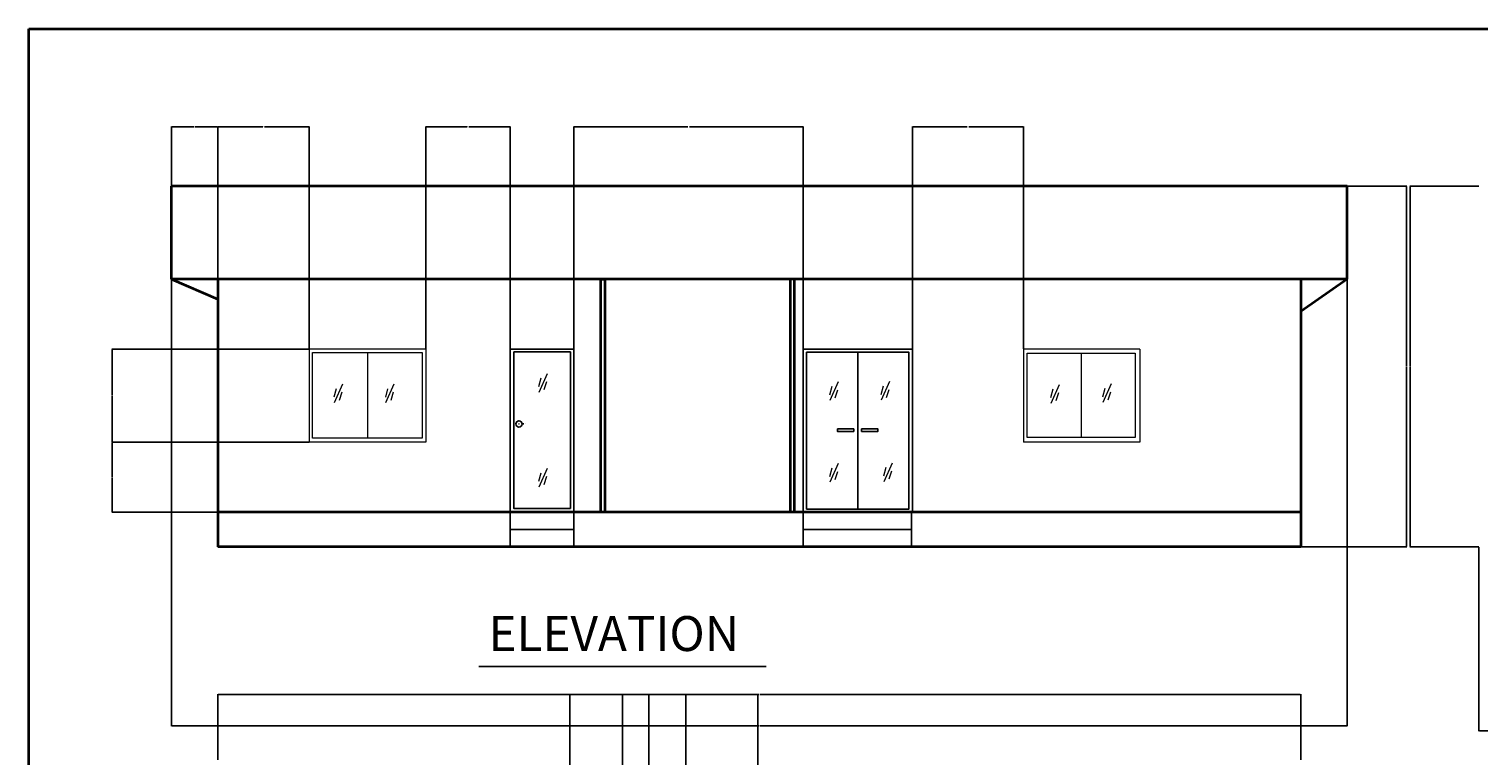
# Model space of a CAD drawing. Units: inches. Extents: x 2215 to 3724, y 1009 to 2124.
# Tile 7 of 11: x 2215 to 2963, y 1750 to 2124. Entities that reach past the tile are written whole.
import ezdxf

# ---------------------------------------------------------------- set-up
doc = ezdxf.new("R2010")
doc.units = ezdxf.units.IN
for name, color, linetype, lineweight in [('A-ANNO-DIMS', 2, 'Continuous', 18), ('A-ANNO-TEXT', 7, 'Continuous', 25), ('A-ANNO-TTLB', 7, 'Continuous', 35), ('A-DOOR', 3, 'Continuous', 25), ('A-ELEV', 7, 'Continuous', 35), ('A-FLOR-STRS', 7, 'Continuous', 25), ('A-GLAZ', 4, 'Continuous', 18)]:
    doc.layers.add(name, color=color, linetype=linetype, lineweight=lineweight)
doc.styles.get("Standard").update_dxf_attribs({"font": 'arial.ttf'})
doc.dimstyles.get("Standard").update_dxf_attribs({"dimtxt": 0.18, "dimasz": 0.18, "dimexe": 0.18, "dimexo": 0.0625, "dimgap": 0.09, "dimtad": 0, "dimtih": 1, "dimtoh": 1, "dimdec": 4, "dimzin": 0, "dimdsep": 46, "dimtxsty": 'Standard', "dimcen": 0.09, "dimadec": 0, "dimazin": 0, "dimtfac": 1, "dimtdec": 4, "dimtofl": 0, "dimtmove": 0, "dimatfit": 3, "dimfxl": 1, "dimtolj": 1, "dimtzin": 0, "dimarcsym": 0})

# ---------------------------------------------------------------- blocks, each defined once
blk = doc.blocks.new('GLASS-REFLECTION')
for p, q in [((4.44, 9.61), (0.14, 0)), ((1.18, 7.28), (0, 2.85)), ((4.09, 5.42), (2.74, 1.25))]:
    blk.add_line(p, q)
blk = doc.blocks.new('*D87')
at = {"layer": 'A-ANNO-DIMS', "color": 0, "lineweight": -2, "transparency": 16777216}
for p, q in [((2312.84, 1747.56), (2312.84, 1781.28)), ((2313.02, 1781.1), (2591.55, 1781.1)), ((2870.66, 1781.1), (2592.13, 1781.1)), ((2870.84, 1747.56), (2870.84, 1781.28))]:
    blk.add_line(p, q, dxfattribs=at)
at = {"layer": 'A-ANNO-DIMS', "color": 0, "transparency": 16777216}
for points in [[(2313.02, 1781.13), (2313.02, 1781.07), (2312.84, 1781.1)], [(2870.66, 1781.13), (2870.66, 1781.07), (2870.84, 1781.1)]]:
    blk.add_solid(points, dxfattribs=at)
at = {"layer": 'Defpoints', "color": 0, "transparency": 16777216}
for p in [(2870.84, 1781.1), (2312.84, 1747.5), (2870.84, 1747.5)]:
    blk.add_point(p, dxfattribs=at)
at = {"layer": 'A-ANNO-DIMS', "color": 0, "transparency": 16777216, "insert": (2591.84, 1781.1), "char_height": 0.18, "attachment_point": 5}
blk.add_mtext('\\A1;558', dxfattribs=at)
blk = doc.blocks.new('*D104')
at = {"layer": 'A-ANNO-DIMS', "color": 0, "lineweight": -2, "transparency": 16777216}
for p, q in [((2553.99, 1430.08), (2553.99, 1781.28)), ((2554.17, 1781.1), (2572.13, 1781.1)), ((2590.88, 1781.1), (2572.92, 1781.1)), ((2591.06, 1430.08), (2591.06, 1781.28))]:
    blk.add_line(p, q, dxfattribs=at)
at = {"layer": 'A-ANNO-DIMS', "color": 0, "transparency": 16777216}
for points in [[(2554.17, 1781.13), (2554.17, 1781.07), (2553.99, 1781.1)], [(2590.88, 1781.13), (2590.88, 1781.07), (2591.06, 1781.1)]]:
    blk.add_solid(points, dxfattribs=at)
at = {"layer": 'Defpoints', "color": 0, "transparency": 16777216}
for p in [(2591.06, 1781.1), (2553.99, 1430.02), (2591.06, 1430.02)]:
    blk.add_point(p, dxfattribs=at)
at = {"layer": 'A-ANNO-DIMS', "color": 0, "transparency": 16777216, "insert": (2572.53, 1781.1), "char_height": 0.18, "attachment_point": 5}
blk.add_mtext('\\A1;37.07', dxfattribs=at)
blk = doc.blocks.new('*D106')
at = {"layer": 'A-ANNO-DIMS', "color": 0, "lineweight": -2, "transparency": 16777216}
for p, q in [((2494.2, 1391.49), (2494.2, 1781.28)), ((2494.38, 1781.1), (2507.39, 1781.1)), ((2521.19, 1781.1), (2508.18, 1781.1)), ((2521.37, 1401.43), (2521.37, 1781.28))]:
    blk.add_line(p, q, dxfattribs=at)
at = {"layer": 'A-ANNO-DIMS', "color": 0, "transparency": 16777216}
for points in [[(2494.38, 1781.13), (2494.38, 1781.07), (2494.2, 1781.1)], [(2521.19, 1781.13), (2521.19, 1781.07), (2521.37, 1781.1)]]:
    blk.add_solid(points, dxfattribs=at)
at = {"layer": 'Defpoints', "color": 0, "transparency": 16777216}
for p in [(2521.37, 1781.1), (2521.37, 1401.36), (2494.2, 1391.42)]:
    blk.add_point(p, dxfattribs=at)
at = {"layer": 'A-ANNO-DIMS', "color": 0, "transparency": 16777216, "insert": (2507.78, 1781.1), "char_height": 0.18, "attachment_point": 5}
blk.add_mtext('\\A1;27.18', dxfattribs=at)
blk = doc.blocks.new('*D107')
at = {"layer": 'A-ANNO-DIMS', "color": 0, "lineweight": -2, "transparency": 16777216}
for p, q in [((2534.96, 1425.13), (2534.96, 1781.28)), ((2535.14, 1781.1), (2544.02, 1781.1)), ((2553.81, 1781.1), (2544.93, 1781.1)), ((2553.99, 1430.08), (2553.99, 1781.28))]:
    blk.add_line(p, q, dxfattribs=at)
at = {"layer": 'A-ANNO-DIMS', "color": 0, "transparency": 16777216}
for points in [[(2535.14, 1781.13), (2535.14, 1781.07), (2534.96, 1781.1)], [(2553.81, 1781.13), (2553.81, 1781.07), (2553.99, 1781.1)]]:
    blk.add_solid(points, dxfattribs=at)
at = {"layer": 'Defpoints', "color": 0, "transparency": 16777216}
for p in [(2553.99, 1781.1), (2553.99, 1430.02), (2534.96, 1425.07)]:
    blk.add_point(p, dxfattribs=at)
at = {"layer": 'A-ANNO-DIMS', "color": 0, "transparency": 16777216, "insert": (2544.48, 1781.1), "char_height": 0.18, "attachment_point": 5}
blk.add_mtext('\\A1;19.027', dxfattribs=at)
blk = doc.blocks.new('*D108')
at = {"layer": 'A-ANNO-DIMS', "color": 0, "lineweight": -2, "transparency": 16777216}
for p, q in [((2288.84, 1995.17), (2288.84, 1764.87)), ((2894.84, 1995.17), (2894.84, 1764.87)), ((2289.02, 1765.05), (2591.55, 1765.05)), ((2894.66, 1765.05), (2592.13, 1765.05))]:
    blk.add_line(p, q, dxfattribs=at)
at = {"layer": 'A-ANNO-DIMS', "color": 0, "transparency": 16777216}
for points in [[(2289.02, 1765.08), (2289.02, 1765.02), (2288.84, 1765.05)], [(2894.66, 1765.08), (2894.66, 1765.02), (2894.84, 1765.05)]]:
    blk.add_solid(points, dxfattribs=at)
at = {"layer": 'Defpoints', "color": 0, "transparency": 16777216}
for p in [(2288.84, 1995.24), (2894.84, 1995.24), (2894.84, 1765.05)]:
    blk.add_point(p, dxfattribs=at)
at = {"layer": 'A-ANNO-DIMS', "color": 0, "transparency": 16777216, "insert": (2591.84, 1765.05), "char_height": 0.18, "attachment_point": 5}
blk.add_mtext('\\A1;606', dxfattribs=at)
blk = doc.blocks.new('*D109')
at = {"layer": 'A-ANNO-DIMS', "color": 0, "lineweight": -2, "transparency": 16777216}
for p, q in [((2894.9, 2043.24), (2925.57, 2043.24)), ((2925.39, 2043.06), (2925.39, 1950.42)), ((2925.39, 1857.42), (2925.39, 1950.06)), ((2870.9, 1857.24), (2925.57, 1857.24))]:
    blk.add_line(p, q, dxfattribs=at)
at = {"layer": 'A-ANNO-DIMS', "color": 0, "transparency": 16777216}
for points in [[(2925.36, 2043.06), (2925.42, 2043.06), (2925.39, 2043.24)], [(2925.36, 1857.42), (2925.42, 1857.42), (2925.39, 1857.24)]]:
    blk.add_solid(points, dxfattribs=at)
at = {"layer": 'Defpoints', "color": 0, "transparency": 16777216}
for p in [(2894.84, 2043.24), (2870.84, 1857.24), (2925.39, 1857.24)]:
    blk.add_point(p, dxfattribs=at)
at = {"layer": 'A-ANNO-DIMS', "color": 0, "transparency": 16777216, "insert": (2925.39, 1950.24), "char_height": 0.18, "attachment_point": 5}
blk.add_mtext('\\A1;186', dxfattribs=at)
blk = doc.blocks.new('*D110')
at = {"layer": 'A-ANNO-DIMS', "color": 0, "lineweight": -2, "transparency": 16777216}
for p, q in [((2288.84, 1995.3), (2288.84, 2073.97)), ((2289.02, 2073.79), (2300.62, 2073.79)), ((2312.66, 2073.79), (2301.06, 2073.79)), ((2312.84, 1995.3), (2312.84, 2073.97))]:
    blk.add_line(p, q, dxfattribs=at)
at = {"layer": 'A-ANNO-DIMS', "color": 0, "transparency": 16777216}
for points in [[(2289.02, 2073.82), (2289.02, 2073.76), (2288.84, 2073.79)], [(2312.66, 2073.82), (2312.66, 2073.76), (2312.84, 2073.79)]]:
    blk.add_solid(points, dxfattribs=at)
at = {"layer": 'Defpoints', "color": 0, "transparency": 16777216}
for p in [(2312.84, 2073.79), (2288.84, 1995.24), (2312.84, 1995.24)]:
    blk.add_point(p, dxfattribs=at)
at = {"layer": 'A-ANNO-DIMS', "color": 0, "transparency": 16777216, "insert": (2300.84, 2073.79), "char_height": 0.18, "attachment_point": 5}
blk.add_mtext('\\A1;24', dxfattribs=at)
blk = doc.blocks.new('*D111')
at = {"layer": 'A-ANNO-DIMS', "color": 0, "lineweight": -2, "transparency": 16777216}
for p, q in [((2312.84, 1995.3), (2312.84, 2073.97)), ((2313.02, 2073.79), (2335.97, 2073.79)), ((2359.72, 2073.79), (2336.77, 2073.79)), ((2359.9, 1959.3), (2359.9, 2073.97))]:
    blk.add_line(p, q, dxfattribs=at)
at = {"layer": 'A-ANNO-DIMS', "color": 0, "transparency": 16777216}
for points in [[(2313.02, 2073.82), (2313.02, 2073.76), (2312.84, 2073.79)], [(2359.72, 2073.82), (2359.72, 2073.76), (2359.9, 2073.79)]]:
    blk.add_solid(points, dxfattribs=at)
at = {"layer": 'Defpoints', "color": 0, "transparency": 16777216}
for p in [(2359.9, 2073.79), (2312.84, 1995.24), (2359.9, 1959.24)]:
    blk.add_point(p, dxfattribs=at)
at = {"layer": 'A-ANNO-DIMS', "color": 0, "transparency": 16777216, "insert": (2336.37, 2073.79), "char_height": 0.18, "attachment_point": 5}
blk.add_mtext('\\A1;47.06', dxfattribs=at)
blk = doc.blocks.new('*D112')
at = {"layer": 'A-ANNO-DIMS', "color": 0, "lineweight": -2, "transparency": 16777216}
for p, q in [((2419.9, 1959.3), (2419.9, 2073.97)), ((2420.08, 2073.79), (2441.3, 2073.79)), ((2463.3, 2073.79), (2442.09, 2073.79)), ((2463.48, 1959.3), (2463.48, 2073.97))]:
    blk.add_line(p, q, dxfattribs=at)
at = {"layer": 'A-ANNO-DIMS', "color": 0, "transparency": 16777216}
for points in [[(2420.08, 2073.82), (2420.08, 2073.76), (2419.9, 2073.79)], [(2463.3, 2073.82), (2463.3, 2073.76), (2463.48, 2073.79)]]:
    blk.add_solid(points, dxfattribs=at)
at = {"layer": 'Defpoints', "color": 0, "transparency": 16777216}
for p in [(2463.48, 2073.79), (2419.9, 1959.24), (2463.48, 1959.24)]:
    blk.add_point(p, dxfattribs=at)
at = {"layer": 'A-ANNO-DIMS', "color": 0, "transparency": 16777216, "insert": (2441.69, 2073.79), "char_height": 0.18, "attachment_point": 5}
blk.add_mtext('\\A1;43.58', dxfattribs=at)
blk = doc.blocks.new('*D113')
at = {"layer": 'A-ANNO-DIMS', "color": 0, "lineweight": -2, "transparency": 16777216}
for p, q in [((2496.28, 1959.3), (2496.28, 2073.97)), ((2496.46, 2073.79), (2554.91, 2073.79)), ((2614.27, 2073.79), (2555.82, 2073.79)), ((2614.45, 1959.3), (2614.45, 2073.97))]:
    blk.add_line(p, q, dxfattribs=at)
at = {"layer": 'A-ANNO-DIMS', "color": 0, "transparency": 16777216}
for points in [[(2496.46, 2073.82), (2496.46, 2073.76), (2496.28, 2073.79)], [(2614.27, 2073.82), (2614.27, 2073.76), (2614.45, 2073.79)]]:
    blk.add_solid(points, dxfattribs=at)
at = {"layer": 'Defpoints', "color": 0, "transparency": 16777216}
for p in [(2614.45, 2073.79), (2496.28, 1959.24), (2614.45, 1959.24)]:
    blk.add_point(p, dxfattribs=at)
at = {"layer": 'A-ANNO-DIMS', "color": 0, "transparency": 16777216, "insert": (2555.36, 2073.79), "char_height": 0.18, "attachment_point": 5}
blk.add_mtext('\\A1;118.18', dxfattribs=at)
blk = doc.blocks.new('*D114')
at = {"layer": 'A-ANNO-DIMS', "color": 0, "lineweight": -2, "transparency": 16777216}
for p, q in [((2670.71, 1959.3), (2670.71, 2073.97)), ((2670.89, 2073.79), (2698.95, 2073.79)), ((2727.8, 2073.79), (2699.74, 2073.79)), ((2727.98, 1959.3), (2727.98, 2073.97))]:
    blk.add_line(p, q, dxfattribs=at)
at = {"layer": 'A-ANNO-DIMS', "color": 0, "transparency": 16777216}
for points in [[(2670.89, 2073.82), (2670.89, 2073.76), (2670.71, 2073.79)], [(2727.8, 2073.82), (2727.8, 2073.76), (2727.98, 2073.79)]]:
    blk.add_solid(points, dxfattribs=at)
at = {"layer": 'Defpoints', "color": 0, "transparency": 16777216}
for p in [(2727.98, 2073.79), (2670.71, 1959.24), (2727.98, 1959.24)]:
    blk.add_point(p, dxfattribs=at)
at = {"layer": 'A-ANNO-DIMS', "color": 0, "transparency": 16777216, "insert": (2699.35, 2073.79), "char_height": 0.18, "attachment_point": 5}
blk.add_mtext('\\A1;57.27', dxfattribs=at)
blk = doc.blocks.new('*D115')
at = {"layer": 'A-ANNO-DIMS', "color": 0, "lineweight": -2, "transparency": 16777216}
for p, q in [((2359.84, 1911.24), (2258.11, 1911.24)), ((2258.29, 1911.06), (2258.29, 1893.42)), ((2258.29, 1875.42), (2258.29, 1893.06)), ((2312.78, 1875.24), (2258.11, 1875.24))]:
    blk.add_line(p, q, dxfattribs=at)
at = {"layer": 'A-ANNO-DIMS', "color": 0, "transparency": 16777216}
for points in [[(2258.26, 1911.06), (2258.32, 1911.06), (2258.29, 1911.24)], [(2258.26, 1875.42), (2258.32, 1875.42), (2258.29, 1875.24)]]:
    blk.add_solid(points, dxfattribs=at)
at = {"layer": 'Defpoints', "color": 0, "transparency": 16777216}
for p in [(2258.29, 1911.24), (2359.9, 1911.24), (2312.84, 1875.24)]:
    blk.add_point(p, dxfattribs=at)
at = {"layer": 'A-ANNO-DIMS', "color": 0, "transparency": 16777216, "insert": (2258.29, 1893.24), "char_height": 0.18, "attachment_point": 5}
blk.add_mtext('\\A1;36', dxfattribs=at)
blk = doc.blocks.new('*D116')
at = {"layer": 'A-ANNO-DIMS', "color": 0, "lineweight": -2, "transparency": 16777216}
for p, q in [((2359.84, 1959.24), (2258.11, 1959.24)), ((2258.29, 1959.06), (2258.29, 1935.42)), ((2258.29, 1911.42), (2258.29, 1935.06)), ((2359.84, 1911.24), (2258.11, 1911.24))]:
    blk.add_line(p, q, dxfattribs=at)
at = {"layer": 'A-ANNO-DIMS', "color": 0, "transparency": 16777216}
for points in [[(2258.26, 1959.06), (2258.32, 1959.06), (2258.29, 1959.24)], [(2258.26, 1911.42), (2258.32, 1911.42), (2258.29, 1911.24)]]:
    blk.add_solid(points, dxfattribs=at)
at = {"layer": 'Defpoints', "color": 0, "transparency": 16777216}
for p in [(2258.29, 1959.24), (2359.9, 1959.24), (2359.9, 1911.24)]:
    blk.add_point(p, dxfattribs=at)
at = {"layer": 'A-ANNO-DIMS', "color": 0, "transparency": 16777216, "insert": (2258.29, 1935.24), "char_height": 0.18, "attachment_point": 5}
blk.add_mtext('\\A1;48', dxfattribs=at)
blk = doc.blocks.new('*D117')
at = {"layer": 'A-ANNO-DIMS', "color": 0, "lineweight": -2, "transparency": 16777216}
for p, q in [((2962.74, 1857.17), (2962.74, 1762.29)), ((3520.74, 1857.17), (3520.74, 1762.29)), ((2962.92, 1762.47), (3241.45, 1762.47)), ((3520.56, 1762.47), (3242.03, 1762.47))]:
    blk.add_line(p, q, dxfattribs=at)
at = {"layer": 'A-ANNO-DIMS', "color": 0, "transparency": 16777216}
for points in [[(2962.92, 1762.5), (2962.92, 1762.44), (2962.74, 1762.47)], [(3520.56, 1762.5), (3520.56, 1762.44), (3520.74, 1762.47)]]:
    blk.add_solid(points, dxfattribs=at)
at = {"layer": 'Defpoints', "color": 0, "transparency": 16777216}
for p in [(2962.74, 1857.24), (3520.74, 1857.24), (3520.74, 1762.47)]:
    blk.add_point(p, dxfattribs=at)
at = {"layer": 'A-ANNO-DIMS', "color": 0, "transparency": 16777216, "insert": (3241.74, 1762.47), "char_height": 0.18, "attachment_point": 5}
blk.add_mtext('\\A1;558', dxfattribs=at)
blk = doc.blocks.new('*D118')
at = {"layer": 'A-ANNO-DIMS', "color": 0, "lineweight": -2, "transparency": 16777216}
for p, q in [((2962.68, 2043.24), (2927.06, 2043.24)), ((2927.24, 2043.06), (2927.24, 1950.42)), ((2927.24, 1857.42), (2927.24, 1950.06)), ((2962.68, 1857.24), (2927.06, 1857.24))]:
    blk.add_line(p, q, dxfattribs=at)
at = {"layer": 'A-ANNO-DIMS', "color": 0, "transparency": 16777216}
for points in [[(2927.21, 2043.06), (2927.27, 2043.06), (2927.24, 2043.24)], [(2927.21, 1857.42), (2927.27, 1857.42), (2927.24, 1857.24)]]:
    blk.add_solid(points, dxfattribs=at)
at = {"layer": 'Defpoints', "color": 0, "transparency": 16777216}
for p in [(2927.24, 2043.24), (2962.74, 2043.24), (2962.74, 1857.24)]:
    blk.add_point(p, dxfattribs=at)
at = {"layer": 'A-ANNO-DIMS', "color": 0, "transparency": 16777216, "insert": (2927.24, 1950.24), "char_height": 0.18, "attachment_point": 5}
blk.add_mtext('\\A1;186', dxfattribs=at)
blk = doc.blocks.new('*D129')
at = {"layer": 'A-ANNO-DIMS', "color": 0, "lineweight": -2, "transparency": 16777216}
for p, q in [((2467.88, 1920.66), (2468.06, 1920.66)), ((2467.97, 1920.57), (2467.97, 1920.75)), ((2470.54, 1920.66), (2469.76, 1920.66))]:
    blk.add_line(p, q, dxfattribs=at)
at = {"layer": 'A-ANNO-DIMS', "color": 0, "transparency": 16777216}
blk.add_solid([(2469.76, 1920.69), (2469.76, 1920.63), (2469.58, 1920.66)], dxfattribs=at)
at = {"layer": 'Defpoints', "color": 0, "transparency": 16777216}
for p in [(2466.35, 1920.66), (2469.58, 1920.66)]:
    blk.add_point(p, dxfattribs=at)
at = {"layer": 'A-ANNO-DIMS', "color": 0, "transparency": 16777216, "insert": (2471.03, 1920.66), "char_height": 0.18, "attachment_point": 5}
blk.add_mtext('\\A1;∅3.223', dxfattribs=at)

msp = doc.modelspace()

# ---------------------------------------------------------------- linework, layer by layer
at = {"layer": 'A-ANNO-TEXT'}
for p, q in [((2447.3483, 1795.6042), (2454.1918, 1795.6042)), ((2454.1918, 1795.6042), (2595.4468, 1795.6042))]:
    msp.add_line(p, q, dxfattribs=at)
at = {"layer": 'A-ANNO-TTLB'}
msp.add_lwpolyline([(2215.4438, 2124.2681), (3723.6589, 2124.2681), (3723.6589, 1008.7935), (2215.4438, 1008.7935)], close=True, dxfattribs=at)
at = {"layer": 'A-DOOR'}
for p, q in [((2463.4826, 1959.2374), (2463.4826, 1875.2374)), ((2463.4826, 1959.2374), (2463.4826, 1875.2374)), ((2496.2773, 1959.2374), (2463.4826, 1959.2374)), ((2496.2773, 1959.2374), (2496.2773, 1875.2374)), ((2614.4526, 1959.2374), (2614.4526, 1875.2374)), ((2670.7119, 1959.2374), (2614.4526, 1959.2374)), ((2670.7119, 1959.2374), (2670.7119, 1875.2374)), ((2642.5672, 1957.6155), (2642.5672, 1876.7284))]:
    msp.add_line(p, q, dxfattribs=at)
for points in [[(2465.3143, 1957.8136), (2494.4737, 1957.8136), (2494.4737, 1877.1133), (2465.3143, 1877.1133)], [(2616.2329, 1957.6155), (2668.9016, 1957.6155), (2668.9016, 1876.7284), (2616.2329, 1876.7284)], [(2632.1099, 1918.1001), (2640.483, 1918.1001), (2640.483, 1916.8283), (2632.1099, 1916.8283)], [(2644.571, 1918.1001), (2652.9441, 1918.1001), (2652.9441, 1916.8283), (2644.571, 1916.8283)]]:
    msp.add_lwpolyline(points, close=True, dxfattribs=at)
msp.add_circle((2467.9651, 1920.659), 1.6114, dxfattribs=at)
at = {"layer": 'A-ELEV'}
for p, q in [((2894.841, 2043.2374), (2288.841, 2043.2374)), ((2288.841, 1995.2374), (2288.841, 2043.2374)), ((2894.841, 1995.2374), (2894.841, 2043.2374)), ((2894.841, 1995.2374), (2288.841, 1995.2374)), ((2288.841, 1995.2374), (2312.841, 1984.8972)), ((2312.841, 1995.2374), (2312.841, 1857.2374)), ((2510.1842, 1875.2374), (2510.1842, 1995.2374)), ((2510.1842, 1995.2374), (2511.1842, 1995.2374)), ((2511.1842, 1995.2374), (2512.1842, 1995.2374)), ((2512.1842, 1995.2374), (2512.1842, 1875.2374)), ((2607.841, 1875.2374), (2607.841, 1995.2374)), ((2607.841, 1995.2374), (2607.841, 1995.2374)), ((2609.841, 1995.2374), (2609.841, 1875.2374)), ((2870.841, 1995.2374), (2870.841, 1857.2374)), ((2894.841, 1995.2374), (2870.841, 1978.5463)), ((2870.841, 1875.2374), (2312.841, 1875.2374)), ((2609.841, 1875.2374), (2607.841, 1875.2374)), ((2870.841, 1857.2374), (2312.841, 1857.2374))]:
    msp.add_line(p, q, dxfattribs=at)
at = {"layer": 'A-FLOR-STRS'}
for p, q in [((2463.4826, 1866.2374), (2496.2527, 1866.2374)), ((2670.2864, 1866.2374), (2614.4526, 1866.2374))]:
    msp.add_line(p, q, dxfattribs=at)
for points in [[(2463.4826, 1875.2374), (2496.2527, 1875.2374), (2496.2527, 1857.2374), (2463.4826, 1857.2374)], [(2614.4526, 1875.2374), (2670.2864, 1875.2374), (2670.2864, 1857.2374), (2614.4526, 1857.2374)]]:
    msp.add_lwpolyline(points, close=True, dxfattribs=at)
at = {"layer": 'A-GLAZ'}
for p, q in [((2359.9027, 1959.2374), (2359.9027, 1911.2374)), ((2419.9027, 1959.2374), (2359.9027, 1959.2374)), ((2419.9027, 1959.2374), (2419.9027, 1911.2374)), ((2727.9846, 1959.2374), (2727.9846, 1911.2374)), ((2787.9846, 1959.2374), (2727.9846, 1959.2374)), ((2787.9846, 1959.2374), (2787.9846, 1911.2374)), ((2389.8676, 1957.4314), (2389.8676, 1913.2638)), ((2757.6988, 1957.1381), (2757.6988, 1913.6384)), ((2419.9027, 1911.2374), (2359.9027, 1911.2374)), ((2787.9846, 1911.2374), (2727.9846, 1911.2374))]:
    msp.add_line(p, q, dxfattribs=at)
for points in [[(2361.6117, 1957.4314), (2418.1235, 1957.4314), (2418.1235, 1913.2638), (2361.6117, 1913.2638)], [(2729.866, 1957.1381), (2785.5316, 1957.1381), (2785.5316, 1913.6384), (2729.866, 1913.6384)]]:
    msp.add_lwpolyline(points, close=True, dxfattribs=at)

# ---------------------------------------------------------------- block references
for p in [(2478.104, 1936.9115), (2372.5016, 1931.5518), (2399.1124, 1931.5518), (2628.002, 1932.7222), (2654.5241, 1932.8395), (2741.9342, 1931.2566), (2768.728, 1931.658), (2628.002, 1890.6093), (2655.815, 1890.8664), (2478.104, 1888.0622)]:
    msp.add_blockref('GLASS-REFLECTION', p, dxfattribs=at)

# ---------------------------------------------------------------- texts
at = {"layer": 'A-ANNO-TEXT', "insert": (2452.2682, 1821.5765), "char_height": 18, "attachment_point": 1}
msp.add_mtext_dynamic_manual_height_columns('ELEVATION', width=452.985586, gutter_width=12.5, heights=[0], dxfattribs=at)

# ---------------------------------------------------------------- dimensions: what is measured, and where the dimension line sits
at = {"layer": 'A-ANNO-DIMS'}
for base, p1, p2, override, picture, middle in [((2312.841, 2073.7874), (2288.841, 1995.2374), (2312.841, 1995.2374), {"dimdec": 0, "dimlfac": 1, "dimrnd": 0, "dimzin": 0, "dimdsep": 46, "dimlunit": 2}, '*D110', (2300.841, 2073.7874)), ((2359.9027, 2073.7874), (2312.841, 1995.2374), (2359.9027, 1959.2374), {"dimdec": 2, "dimlfac": 1, "dimrnd": 0, "dimzin": 0, "dimdsep": 46, "dimlunit": 2}, '*D111', (2336.3718, 2073.7874)), ((2463.4826, 2073.7874), (2419.9027, 1959.2374), (2463.4826, 1959.2374), {"dimdec": 2, "dimlfac": 1, "dimrnd": 0, "dimzin": 0, "dimdsep": 46, "dimlunit": 2}, '*D112', (2441.6926, 2073.7874)), ((2614.4526, 2073.7874), (2496.2773, 1959.2374), (2614.4526, 1959.2374), {"dimdec": 2, "dimlfac": 1, "dimrnd": 0, "dimzin": 0, "dimdsep": 46, "dimlunit": 2}, '*D113', (2555.365, 2073.7874)), ((2727.9846, 2073.7874), (2670.7119, 1959.2374), (2727.9846, 1959.2374), {"dimdec": 2, "dimlfac": 1, "dimrnd": 0, "dimzin": 0, "dimdsep": 46, "dimlunit": 2}, '*D114', (2699.3483, 2073.7874)), ((2894.841, 1765.0542), (2288.841, 1995.2374), (2894.841, 1995.2374), {"dimdec": 0, "dimlfac": 1, "dimrnd": 0, "dimzin": 0, "dimdsep": 46, "dimlunit": 2}, '*D108', (2591.841, 1765.0542)), ((3520.7432, 1762.4722), (2962.7432, 1857.2374), (3520.7432, 1857.2374), {"dimdec": 0, "dimlfac": 1, "dimrnd": 0, "dimzin": 0, "dimdsep": 46, "dimlunit": 2}, '*D117', (3241.7432, 1762.4722)), ((2870.841, 1781.0969), (2312.841, 1747.4969), (2870.841, 1747.4969), {"dimdec": 0, "dimlfac": 1, "dimrnd": 0, "dimzin": 0, "dimdsep": 46, "dimlunit": 2}, '*D87', (2591.841, 1781.0969)), ((2521.3728, 1781.0969), (2494.1952, 1391.4229), (2521.3728, 1401.3639), {"dimdec": 2, "dimlfac": 1, "dimrnd": 0, "dimzin": 0, "dimdsep": 46, "dimlunit": 2}, '*D106', (2507.784, 1781.0969)), ((2553.9914, 1781.0969), (2534.9648, 1425.0681), (2553.9914, 1430.018), {"dimdec": 3, "dimlfac": 1, "dimrnd": 0, "dimzin": 0, "dimdsep": 46, "dimlunit": 2}, '*D107', (2544.4781, 1781.0969)), ((2591.0617, 1781.0969), (2553.9914, 1430.018), (2591.0617, 1430.018), {"dimdec": 2, "dimlfac": 1, "dimrnd": 0, "dimzin": 0, "dimdsep": 46, "dimlunit": 2}, '*D104', (2572.5266, 1781.0969))]:
    dim = msp.add_linear_dim(base=base, p1=p1, p2=p2, dimstyle='Standard', override=override, dxfattribs=at)
    dim.commit()
    dim.dimension.update_dxf_attribs({"geometry": picture, "text_midpoint": middle})
for base, p1, p2, picture, middle in [((2925.391, 1857.2374), (2894.841, 2043.2374), (2870.841, 1857.2374), '*D109', (2925.391, 1950.2374)), ((2927.2432, 2043.2374), (2962.7432, 1857.2374), (2962.7432, 2043.2374), '*D118', (2927.2432, 1950.2374)), ((2258.291, 1959.2374), (2359.9027, 1911.2374), (2359.9027, 1959.2374), '*D116', (2258.291, 1935.2374)), ((2258.291, 1911.2374), (2312.841, 1875.2374), (2359.9027, 1911.2374), '*D115', (2258.291, 1893.2374))]:
    dim = msp.add_linear_dim(base=base, p1=p1, p2=p2, angle=90, dimstyle='Standard', override={"dimdec": 0, "dimlfac": 1, "dimrnd": 0, "dimzin": 0, "dimdsep": 46, "dimlunit": 2}, dxfattribs=at)
    dim.commit()
    dim.dimension.update_dxf_attribs({"geometry": picture, "text_midpoint": middle})
dim = msp.add_diameter_dim_2p(p1=(2466.3537, 1920.659), p2=(2469.5765, 1920.659), dimstyle='Standard', override={"dimdec": 3, "dimlfac": 1, "dimrnd": 0, "dimzin": 0, "dimdsep": 46, "dimlunit": 2}, dxfattribs=at)
dim.commit()
dim.dimension.update_dxf_attribs({"geometry": '*D129', "text_midpoint": (2470.5433, 1920.659), "dimtype": 163})

doc.saveas('drawing.dxf')
